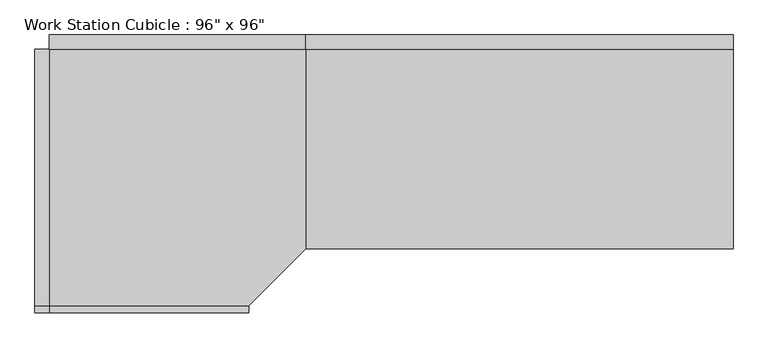
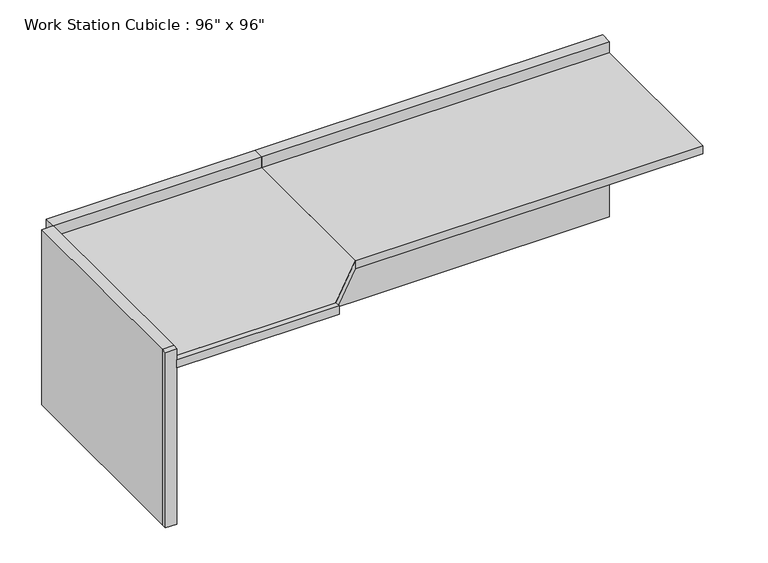
"""IFC4 building model written with IfcOpenShell, lengths in millimetres: furniture geometry."""

from ifc_helpers import new_model, si_unit, frame, origin, origin_with_axes, place, context, project, spatial, polyline, outline, extrude, source, transform, mapped, element, save


def furniture_f408c91c(model_context):
    return source(origin(), model_context, "Body", "SweptSolid", [
        extrude(outline(polyline([(-80.9317522, -545.8230076), (833.4682478, -545.8230076), (833.4682478, -1257.0230076), (630.2682478, -1460.2230076), (-80.9317522, -1460.2230076), (-80.9317522, -545.8230076)])), frame((0.0, 0.0, 723.9), z_axis=(0.0, 0.0, 1.0), x_axis=(1.0, 0.0, 0.0)), (0.0, 0.0, 1.0), 38.1),
        extrude(outline(polyline([(630.2682478, -1485.6230076), (-80.9317522, -1485.6230076), (-80.9317522, -1460.2230076), (630.2682478, -1460.2230076), (630.2682478, -1485.6230076)])), frame((0.0, 0.0, 723.9), z_axis=(0.0, 0.0, 1.0), x_axis=(1.0, 0.0, 0.0)), (0.0, 0.0, 1.0), 38.1),
        extrude(outline(polyline([(2357.4682478, -1257.0230076), (833.4682478, -1257.0230076), (833.4682478, -545.8230076), (2357.4682478, -545.8230076), (2357.4682478, -1257.0230076)])), frame((0.0, 0.0, 723.9), z_axis=(0.0, 0.0, 1.0), x_axis=(1.0, 0.0, 0.0)), (0.0, 0.0, 1.0), 38.1),
        extrude(outline(polyline([(2357.4682478, -545.8230076), (833.4682478, -545.8230076), (833.4682478, -495.0230076), (2357.4682478, -495.0230076), (2357.4682478, -545.8230076)])), origin_with_axes(), (0.0, 0.0, 1.0), 812.8),
        extrude(outline(polyline([(833.4682478, -545.8230076), (-80.9317522, -545.8230076), (-80.9317522, -495.0230076), (833.4682478, -495.0230076), (833.4682478, -545.8230076)])), origin_with_axes(), (0.0, 0.0, 1.0), 812.8),
        extrude(outline(polyline([(-80.9317522, -1460.2230076), (-131.7317522, -1460.2230076), (-131.7317522, -545.8230076), (-80.9317522, -545.8230076), (-80.9317522, -1460.2230076)])), origin_with_axes(), (0.0, 0.0, 1.0), 812.8),
        extrude(outline(polyline([(-80.9317522, -1485.6230076), (-131.7317522, -1485.6230076), (-131.7317522, -1460.2230076), (-80.9317522, -1460.2230076), (-80.9317522, -1485.6230076)])), origin_with_axes(), (0.0, 0.0, 1.0), 812.8),
    ])


if __name__ == "__main__":
    model = new_model("IFC4")
    model_context = context("Model", 3, world=origin())
    ifc_project = project(units=[si_unit("LENGTHUNIT", "METRE", prefix="MILLI")], contexts=[model_context])
    site = spatial("IfcSite", under=ifc_project)
    building = spatial("IfcBuilding", under=site)
    placement = place(None, origin())
    furniture_shape = furniture_f408c91c(model_context)
    element("IfcFurniture", 1, ObjectType="Work Station Cubicle : 96\" x 96\"", at=placement, inside=building, context=model_context, shape_type="MappedRepresentation", body=[
        mapped(furniture_shape, transform((0.0, 0.0, 0.0), x_axis=(1.0, 0.0, 0.0), y_axis=(0.0, 1.0, 0.0), z_axis=(0.0, 0.0, 1.0))),
    ])
    save(model, "model.ifc")

# Revit data of these elements
# Type "Work Station Cubicle : 96\" x 96\""
#   Assembly Code = "E2020"
#   Desktop Height = 2' - 6"
#   Desktop1 Width = 2' - 4"
#   Desktop2 Width = 2' - 4"
#   Panel Height = 2' - 8"
#   Panel1 Length = 0' - 1"
#   Panel2 Length = 5' - 0"
#   Cube Panel Material = Textile - Light Gray
#   Work Top Material = Laminate, Ivory, Matte
#   Default Elevation = 0
# Element 1 (IfcFurniture, "Work Station Cubicle : 96\" x 96\"")
#   Materials on its faces: "Textile - Light Gray", "Laminate, Ivory, Matte"
# Materials
#   "Textile - Light Gray": class "Fabric", colour RGB 204 204 204, transparency 0
#   "Laminate, Ivory, Matte": class "Plastic", colour RGB 247 247 239, transparency 0, Description = "Plastic Laminate - Ivory, Matte", Cost = 0
